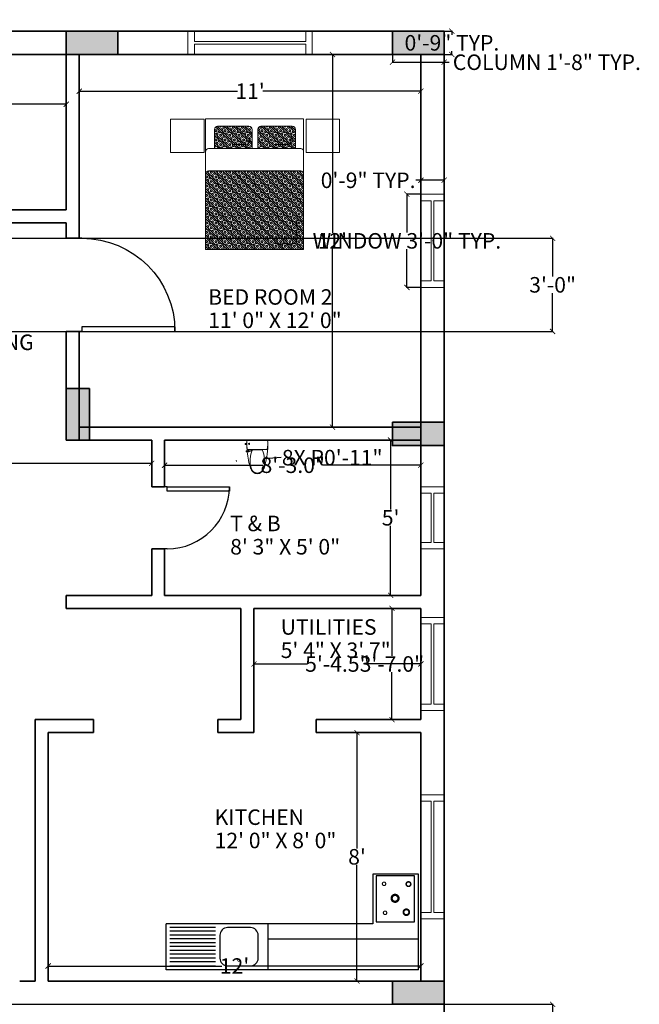
# Model space of a CAD drawing. Units: inches. Extents: x 560 to 1118, y 291 to 1226.
# Tile 4 of 4: x 878 to 1118, y 804 to 1184. Entities that reach past the tile are written whole.
import ezdxf

# ---------------------------------------------------------------- set-up
doc = ezdxf.new("R2010")
doc.units = ezdxf.units.IN
doc.header["$MEASUREMENT"] = 0
for name, color, linetype, lineweight in [('A-ANNO-DIMS', 2, 'Continuous', 13), ('A-AREA-IDEN', 7, 'Continuous', 18), ('A-COLS', 7, 'Continuous', 35), ('A-FLOR-FIXT', 9, 'Continuous', 18), ('DOORS', 4, 'Continuous', 25), ('FURNITURE', 8, 'Continuous', 18), ('WALL', 7, 'Continuous', 35), ('WINDOWS', 80, 'Continuous', 18)]:
    doc.layers.add(name, color=color, linetype=linetype, lineweight=lineweight)
doc.layers.add('DUVAR', color=7, linetype='Continuous')
doc.layers.add('TEFRIS', color=11, linetype='Continuous')
doc.styles.get("Standard").update_dxf_attribs({"font": 'arial.ttf'})
doc.dimstyles.get("Standard").update_dxf_attribs({"dimtxt": 6, "dimasz": 2, "dimexe": 0.18, "dimexo": 0.0625, "dimgap": 0.09, "dimtad": 0, "dimtih": 1, "dimtoh": 1, "dimdec": 1, "dimzin": 0, "dimdsep": 46, "dimlunit": 3, "dimtxsty": 'Standard', "dimblk": 'ARCHTICK', "dimcen": 0.09, "dimadec": 0, "dimazin": 0, "dimtfac": 1, "dimtdec": 1, "dimtofl": 0, "dimtmove": 0, "dimatfit": 3, "dimfxl": 1, "dimtolj": 1, "dimtzin": 0, "dimarcsym": 0})
pattern_1 = [(135, (-1377.70473, -125.71507), (-0.070710678, -0.070710678), []), (135, (-1377.68705, -125.69739), (-0.070710678, -0.070710678), []), (45, (-1377.70473, -125.71507), (-0.070710678, 0.070710678), [-0.025, 0.025]), (45, (-1377.72241, -125.69739), (-0.070710678, 0.070710678), [-0.025, 0.025]), (45, (-1377.74009, -125.67972), (-0.070710678, 0.070710678), [0.025, -0.025]), (45, (-1377.75776, -125.66204), (-0.070710678, 0.070710678), [0.025, -0.025]), (135, (-1377.66938, -125.67972), (-0.070710678, -0.070710678), [0.025, -0.025]), (135, (-1377.6517, -125.66204), (-0.070710678, -0.070710678), [0.025, -0.025])]

# ---------------------------------------------------------------- blocks, each defined once
blk = doc.blocks.new('*U3')
for p, q in [((0, 0), (0, -6)), ((36, 0), (36, -6))]:
    blk.add_line(p, q)
blk.add_lwpolyline([(0, 0), (0, 36), (1.75, 36), (1.75, 0)], close=True)
blk.add_arc((0, 0), 36, 0, 90)
blk = doc.blocks.new('*U4')
for p, q in [((0, 0), (0, -6)), ((24, 0), (24, -6))]:
    blk.add_line(p, q)
blk.add_lwpolyline([(0, 0), (0, 24), (1.75, 24), (1.75, 0)], close=True)
blk.add_arc((0, 0), 24, 0, 90)
blk = doc.blocks.new('_ArchTick')
at = {"color": 0, "linetype": 'ByBlock', "const_width": 0.15}
blk.add_lwpolyline([(-0.5, -0.5), (0.5, 0.5)], dxfattribs=at)
blk = doc.blocks.new('*D8')
at = {"layer": 'A-ANNO-DIMS', "color": 0, "lineweight": -2, "transparency": 16777216}
for p, q in [((761.18, 1149.36), (761.18, 1151.98)), ((761.18, 1151.8), (815.07, 1151.8)), ((896.18, 1151.8), (842.29, 1151.8)), ((896.18, 1149.36), (896.18, 1151.98))]:
    blk.add_line(p, q, dxfattribs=at)
at = {"layer": 'Defpoints', "color": 0, "transparency": 16777216}
for p in [(761.18, 1149.3), (896.18, 1151.8), (896.18, 1149.3)]:
    blk.add_point(p, dxfattribs=at)
at = {"layer": 'A-ANNO-DIMS', "color": 0, "lineweight": -2, "transparency": 16777216, "xscale": 2, "yscale": 2, "zscale": 2, "rotation": 180}
blk.add_blockref('_ArchTick', (761.18, 1151.8), dxfattribs=at)
at = {"layer": 'A-ANNO-DIMS', "color": 0, "lineweight": -2, "transparency": 16777216, "xscale": 2, "yscale": 2, "zscale": 2}
blk.add_blockref('_ArchTick', (896.18, 1151.8), dxfattribs=at)
at = {"layer": 'A-ANNO-DIMS', "color": 0, "transparency": 16777216, "insert": (828.68, 1151.8), "char_height": 6, "attachment_point": 5}
blk.add_mtext('\\A1;11\'-3.0"', dxfattribs=at)
blk = doc.blocks.new('*D10')
at = {"layer": 'A-ANNO-DIMS', "color": 0, "lineweight": -2, "transparency": 16777216}
for p, q in [((1001.94, 1171), (998.82, 1171)), ((999, 1171), (999, 1102.1)), ((999, 1027), (999, 1095.9)), ((1001.94, 1027), (998.82, 1027))]:
    blk.add_line(p, q, dxfattribs=at)
at = {"layer": 'Defpoints', "color": 0, "transparency": 16777216}
for p in [(1002, 1171), (999, 1027), (1002, 1027)]:
    blk.add_point(p, dxfattribs=at)
at = {"layer": 'A-ANNO-DIMS', "color": 0, "lineweight": -2, "transparency": 16777216, "xscale": 2, "yscale": 2, "zscale": 2}
for p, rotation in [((999, 1171), 90), ((999, 1027), 270)]:
    blk.add_blockref('_ArchTick', p, dxfattribs=dict(at, rotation=rotation))
at = {"layer": 'A-ANNO-DIMS', "color": 0, "transparency": 16777216, "insert": (999, 1099), "char_height": 6, "attachment_point": 5}
blk.add_mtext("\\A1;12'", dxfattribs=at)
blk = doc.blocks.new('*D11')
at = {"layer": 'A-ANNO-DIMS', "color": 0, "lineweight": -2, "transparency": 16777216}
for p, q in [((901.18, 1165.24), (901.18, 1156.62)), ((1033.18, 1165.24), (1033.18, 1156.62)), ((901.18, 1156.8), (962.28, 1156.8)), ((1033.18, 1156.8), (972.08, 1156.8))]:
    blk.add_line(p, q, dxfattribs=at)
at = {"layer": 'Defpoints', "color": 0, "transparency": 16777216}
for p in [(901.18, 1165.3), (1033.18, 1165.3), (1033.18, 1156.8)]:
    blk.add_point(p, dxfattribs=at)
at = {"layer": 'A-ANNO-DIMS', "color": 0, "lineweight": -2, "transparency": 16777216, "xscale": 2, "yscale": 2, "zscale": 2, "rotation": 180}
blk.add_blockref('_ArchTick', (901.18, 1156.8), dxfattribs=at)
at = {"layer": 'A-ANNO-DIMS', "color": 0, "lineweight": -2, "transparency": 16777216, "xscale": 2, "yscale": 2, "zscale": 2}
blk.add_blockref('_ArchTick', (1033.18, 1156.8), dxfattribs=at)
at = {"layer": 'A-ANNO-DIMS', "color": 0, "transparency": 16777216, "insert": (967.18, 1156.8), "char_height": 6, "attachment_point": 5}
blk.add_mtext("\\A1;11'", dxfattribs=at)
blk = doc.blocks.new('*D14')
at = {"layer": 'A-ANNO-DIMS', "color": 0, "lineweight": -2, "transparency": 16777216}
for p, q in [((934.18, 1011.86), (934.18, 1012.48)), ((934.18, 1012.3), (972.12, 1012.3)), ((1033.18, 1012.3), (995.24, 1012.3)), ((1033.18, 1011.86), (1033.18, 1012.48))]:
    blk.add_line(p, q, dxfattribs=at)
at = {"layer": 'Defpoints', "color": 0, "transparency": 16777216}
for p in [(934.18, 1012.3), (934.18, 1011.8), (1033.18, 1011.8)]:
    blk.add_point(p, dxfattribs=at)
at = {"layer": 'A-ANNO-DIMS', "color": 0, "lineweight": -2, "transparency": 16777216, "xscale": 2, "yscale": 2, "zscale": 2, "rotation": 180}
blk.add_blockref('_ArchTick', (934.18, 1012.3), dxfattribs=at)
at = {"layer": 'A-ANNO-DIMS', "color": 0, "lineweight": -2, "transparency": 16777216, "xscale": 2, "yscale": 2, "zscale": 2}
blk.add_blockref('_ArchTick', (1033.18, 1012.3), dxfattribs=at)
at = {"layer": 'A-ANNO-DIMS', "color": 0, "transparency": 16777216, "insert": (983.68, 1012.3), "char_height": 6, "attachment_point": 5}
blk.add_mtext('\\A1;8\'-3.0"', dxfattribs=at)
blk = doc.blocks.new('*D15')
at = {"layer": 'A-ANNO-DIMS', "color": 0, "lineweight": -2, "transparency": 16777216}
for p, q in [((1018.56, 1022), (1021.68, 1022)), ((1021.5, 1022), (1021.5, 995.14)), ((1021.5, 962), (1021.5, 988.86)), ((1018.56, 962), (1021.68, 962))]:
    blk.add_line(p, q, dxfattribs=at)
at = {"layer": 'Defpoints', "color": 0, "transparency": 16777216}
for p in [(1018.5, 1022), (1018.5, 962), (1021.5, 962)]:
    blk.add_point(p, dxfattribs=at)
at = {"layer": 'A-ANNO-DIMS', "color": 0, "lineweight": -2, "transparency": 16777216, "xscale": 2, "yscale": 2, "zscale": 2}
for p, rotation in [((1021.5, 1022), 90), ((1021.5, 962), 270)]:
    blk.add_blockref('_ArchTick', p, dxfattribs=dict(at, rotation=rotation))
at = {"layer": 'A-ANNO-DIMS', "color": 0, "transparency": 16777216, "insert": (1021.5, 992), "char_height": 6, "attachment_point": 5}
blk.add_mtext("\\A1;5'", dxfattribs=at)
blk = doc.blocks.new('*D34')
at = {"layer": 'A-ANNO-DIMS', "color": 0, "lineweight": -2, "transparency": 16777216}
for p, q in [((889.18, 818.86), (889.18, 818.98)), ((889.18, 818.8), (956.28, 818.8)), ((1033.18, 818.8), (966.08, 818.8)), ((1033.18, 818.86), (1033.18, 818.98))]:
    blk.add_line(p, q, dxfattribs=at)
at = {"layer": 'Defpoints', "color": 0, "transparency": 16777216}
for p in [(889.18, 818.8), (1033.18, 818.8), (1033.18, 818.8)]:
    blk.add_point(p, dxfattribs=at)
at = {"layer": 'A-ANNO-DIMS', "color": 0, "lineweight": -2, "transparency": 16777216, "xscale": 2, "yscale": 2, "zscale": 2, "rotation": 180}
blk.add_blockref('_ArchTick', (889.18, 818.8), dxfattribs=at)
at = {"layer": 'A-ANNO-DIMS', "color": 0, "lineweight": -2, "transparency": 16777216, "xscale": 2, "yscale": 2, "zscale": 2}
blk.add_blockref('_ArchTick', (1033.18, 818.8), dxfattribs=at)
at = {"layer": 'A-ANNO-DIMS', "color": 0, "transparency": 16777216, "insert": (961.18, 818.8), "char_height": 6, "attachment_point": 5}
blk.add_mtext("\\A1;12'", dxfattribs=at)
blk = doc.blocks.new('*D35')
at = {"layer": 'A-ANNO-DIMS', "color": 0, "lineweight": -2, "transparency": 16777216}
for p, q in [((1008.5, 909), (1008.5, 864.15)), ((1008.56, 909), (1008.68, 909)), ((1008.5, 813), (1008.5, 857.85)), ((1008.56, 813), (1008.68, 813))]:
    blk.add_line(p, q, dxfattribs=at)
at = {"layer": 'Defpoints', "color": 0, "transparency": 16777216}
for p in [(1008.5, 909), (1008.5, 813), (1008.5, 813)]:
    blk.add_point(p, dxfattribs=at)
at = {"layer": 'A-ANNO-DIMS', "color": 0, "lineweight": -2, "transparency": 16777216, "xscale": 2, "yscale": 2, "zscale": 2}
for p, rotation in [((1008.5, 909), 90), ((1008.5, 813), 270)]:
    blk.add_blockref('_ArchTick', p, dxfattribs=dict(at, rotation=rotation))
at = {"layer": 'A-ANNO-DIMS', "color": 0, "transparency": 16777216, "insert": (1008.5, 861), "char_height": 6, "attachment_point": 5}
blk.add_mtext("\\A1;8'", dxfattribs=at)
blk = doc.blocks.new('*D36')
at = {"layer": 'A-ANNO-DIMS', "color": 0, "lineweight": -2, "transparency": 16777216}
for p, q in [((968.68, 935.56), (968.68, 935.68)), ((968.68, 935.5), (989.37, 935.5)), ((1033.18, 935.5), (1012.49, 935.5)), ((1033.18, 935.56), (1033.18, 935.68))]:
    blk.add_line(p, q, dxfattribs=at)
at = {"layer": 'Defpoints', "color": 0, "transparency": 16777216}
for p in [(968.68, 935.5), (1033.18, 935.5), (1033.18, 935.5)]:
    blk.add_point(p, dxfattribs=at)
at = {"layer": 'A-ANNO-DIMS', "color": 0, "lineweight": -2, "transparency": 16777216, "xscale": 2, "yscale": 2, "zscale": 2, "rotation": 180}
blk.add_blockref('_ArchTick', (968.68, 935.5), dxfattribs=at)
at = {"layer": 'A-ANNO-DIMS', "color": 0, "lineweight": -2, "transparency": 16777216, "xscale": 2, "yscale": 2, "zscale": 2}
blk.add_blockref('_ArchTick', (1033.18, 935.5), dxfattribs=at)
at = {"layer": 'A-ANNO-DIMS', "color": 0, "transparency": 16777216, "insert": (1000.93, 935.5), "char_height": 6, "attachment_point": 5}
blk.add_mtext('\\A1;5\'-4.5"', dxfattribs=at)
blk = doc.blocks.new('*D37')
at = {"layer": 'A-ANNO-DIMS', "color": 0, "lineweight": -2, "transparency": 16777216}
for p, q in [((1020.06, 957), (1022.18, 957)), ((1022, 957), (1022, 938.66)), ((1022, 914), (1022, 932.34)), ((1020.06, 914), (1022.18, 914))]:
    blk.add_line(p, q, dxfattribs=at)
at = {"layer": 'Defpoints', "color": 0, "transparency": 16777216}
for p in [(1020, 957), (1020, 914), (1022, 914)]:
    blk.add_point(p, dxfattribs=at)
at = {"layer": 'A-ANNO-DIMS', "color": 0, "lineweight": -2, "transparency": 16777216, "xscale": 2, "yscale": 2, "zscale": 2}
for p, rotation in [((1022, 957), 90), ((1022, 914), 270)]:
    blk.add_blockref('_ArchTick', p, dxfattribs=dict(at, rotation=rotation))
at = {"layer": 'A-ANNO-DIMS', "color": 0, "transparency": 16777216, "insert": (1022, 935.5), "char_height": 6, "attachment_point": 5}
blk.add_mtext('\\A1;3\'-7.0"', dxfattribs=at)
blk = doc.blocks.new('*D39')
at = {"layer": 'A-ANNO-DIMS', "color": 0, "lineweight": -2, "transparency": 16777216}
for p, q in [((728.18, 1015.74), (728.18, 1012.82)), ((728.18, 1013), (815.07, 1013)), ((929.18, 1013), (842.29, 1013)), ((929.18, 1015.74), (929.18, 1012.82))]:
    blk.add_line(p, q, dxfattribs=at)
at = {"layer": 'Defpoints', "color": 0, "transparency": 16777216}
for p in [(728.18, 1015.8), (929.18, 1015.8), (929.18, 1013)]:
    blk.add_point(p, dxfattribs=at)
at = {"layer": 'A-ANNO-DIMS', "color": 0, "lineweight": -2, "transparency": 16777216, "xscale": 2, "yscale": 2, "zscale": 2, "rotation": 180}
blk.add_blockref('_ArchTick', (728.18, 1013), dxfattribs=at)
at = {"layer": 'A-ANNO-DIMS', "color": 0, "lineweight": -2, "transparency": 16777216, "xscale": 2, "yscale": 2, "zscale": 2}
blk.add_blockref('_ArchTick', (929.18, 1013), dxfattribs=at)
at = {"layer": 'A-ANNO-DIMS', "color": 0, "transparency": 16777216, "insert": (828.68, 1013), "char_height": 6, "attachment_point": 5}
blk.add_mtext('\\A1;16\'-9.0"', dxfattribs=at)
blk = doc.blocks.new('MAT-P10')
h = blk.add_hatch()
h.set_pattern_fill('BOX', color=256, scale=0.1, angle=45, style=0)
h.set_pattern_definition(pattern_1)
h.paths.add_polyline_path([(-0.157, 1.46), (0.417, 1.46), (0.417, 1.751, 0.414214), (0.367, 1.801), (-0.107, 1.801, 0.414214), (-0.157, 1.751)])
h.paths.add_polyline_path([(0.505, 1.46), (1.079, 1.46), (1.079, 1.751, 0.414214), (1.029, 1.801), (0.555, 1.801, 0.414214), (0.505, 1.751)])
h = blk.add_hatch()
h.set_pattern_fill('BOX', color=256, scale=0.1, angle=45, style=0)
h.set_pattern_definition(pattern_1)
edge = h.paths.add_edge_path()
edge.add_line((1.205, -0.085), (1.205, 1.062))
edge.add_ellipse((1.161, 1.063), major_axis=(0, 0.0568), ratio=0.776379, start_angle=270, end_angle=360)
edge.add_line((1.161, 1.119), (-0.251, 1.12))
edge.add_ellipse((-0.251, 1.063), major_axis=(0, 0.0568), ratio=0.776379, start_angle=0, end_angle=88.1396)
edge.add_line((-0.295, 1.064), (-0.295, -0.085))
edge.add_line((-0.295, -0.085), (1.205, -0.085))
for p, q in [((-0.251, 1.46), (1.161, 1.46)), ((-0.251, 1.12), (1.161, 1.119)), ((1.102, 0.406), (1.102, 0.057)), ((1.058, 0), (0.775, 0))]:
    blk.add_line(p, q)
for points in [[(-0.83, 1.909), (-0.319, 1.909), (-0.319, 1.398), (-0.83, 1.398)], [(1.205, -0.085), (-0.295, -0.085), (-0.295, 1.915), (1.205, 1.915)], [(1.244, 1.909), (1.755, 1.909), (1.755, 1.398), (1.244, 1.398)]]:
    blk.add_lwpolyline(points, close=True)
for points in [[(0.417, 1.46), (0.417, 1.751, 0.414214), (0.367, 1.801), (-0.107, 1.801, 0.414214), (-0.157, 1.751), (-0.157, 1.46)], [(1.079, 1.46), (1.079, 1.751, 0.414214), (1.029, 1.801), (0.555, 1.801, 0.414214), (0.505, 1.751), (0.505, 1.46)], [(0.37, 1.624), (0.37, 1.571, -0.414214), (0.32, 1.521), (0.111, 1.521)], [(1.012, 1.644), (1.012, 1.571, -0.414214), (0.962, 1.521), (0.753, 1.521)]]:
    blk.add_lwpolyline(points, format="xyb")
at = {"extrusion": (0, 0, -1)}
for centre, start_param, end_param in [((-0.251, 1.404), 4.712389, 6.283185), ((1.161, 1.404), 0, 1.570796), ((-0.251, 1.063), 4.712389, 6.283185), ((1.161, 1.063), 0, 1.570796), ((1.058, 0.057), 1.570796, 3.141593), ((1.058, 0.057), 1.570796, 3.141593)]:
    blk.add_ellipse(centre, major_axis=(0, 0.0568), ratio=0.776379, start_param=start_param, end_param=end_param, dxfattribs=at)
blk = doc.blocks.new('A$C3F871443')
at = {"layer": 'DUVAR'}
blk.add_line((3, 0), (3.3, 0), dxfattribs=at)
at = {"layer": 'TEFRIS'}
for p, q in [((0, 0), (0, -1.25)), ((0, 0), (3.3, 0)), ((1.97, -0.6), (1.97, 0)), ((3.3, 0), (3.3, -0.6)), ((3.253, -0.055), (2.653, -0.055)), ((2.653, -0.105), (3.253, -0.105)), ((2.653, -0.155), (3.253, -0.155)), ((2.653, -0.205), (3.253, -0.205)), ((2.653, -0.255), (3.253, -0.255)), ((2.653, -0.305), (3.253, -0.305)), ((2.653, -0.355), (3.253, -0.355)), ((0, -0.4), (1.97, -0.4)), ((2.653, -0.405), (3.253, -0.405)), ((2.653, -0.455), (3.253, -0.455)), ((2.653, -0.505), (3.253, -0.505)), ((0.6, -0.6), (3.3, -0.6)), ((0.6, -1.25), (0.6, -0.6)), ((2.653, -0.555), (3.253, -0.555)), ((0, -1.25), (0.6, -1.25))]:
    blk.add_line(p, q, dxfattribs=at)
blk.add_lwpolyline([(2.597, -0.452), (2.597, -0.152, 0.414214), (2.497, -0.052), (2.197, -0.052, 0.414214), (2.097, -0.152), (2.097, -0.452, 0.414214), (2.197, -0.552), (2.497, -0.552, 0.414214)], format="xyb", close=True, dxfattribs=at)
for points, const_width in [([(2.349, -0.141, 1), (2.349, -0.111, 1)], 0.01), ([(0.161, -0.791, 1), (0.161, -0.716, 1)], 0.025), ([(0.439, -0.768, 1), (0.439, -0.723, 1)], 0.015), ([(0.308, -0.98, 1), (0.308, -0.89, 1)], 0.03), ([(0.133, -1.151, 1), (0.133, -1.091, 1)], 0.02), ([(0.452, -1.147, 1), (0.452, -1.102, 1)], 0.015)]:
    blk.add_lwpolyline(points, format="xyb", close=True, dxfattribs=dict(at, const_width=const_width))
blk.add_lwpolyline([(0.556, -1.228), (0.556, -0.628), (0.056, -0.628), (0.056, -1.228)], close=True, dxfattribs=at)
blk = doc.blocks.new('toilet-7')
at = {"color": 0, "linetype": 'ByBlock'}
for p, q in [((-0.246, -0.087), (-0.246, -0.107)), ((-0.246, -0.087), (-0.226, -0.087)), ((-0.246, -0.107), (-0.226, -0.107)), ((-0.226, -0.085), (-0.226, -0.11)), ((-0.226, -0.085), (-0.216, -0.085)), ((-0.226, -0.11), (-0.215, -0.11)), ((0.21, -0.02), (-0.21, -0.02)), ((0.199, -0.212), (0.21, -0.164)), ((0.215, -0.068), (0.21, -0.02)), ((0.21, -0.164), (0.215, -0.117)), ((0.215, -0.117), (0.215, -0.068)), ((-0.121, -0.237), (-0.228, -0.237)), ((-0.228, -0.237), (-0.228, -0.26)), ((-0.176, -0.26), (-0.228, -0.26)), ((0.199, -0.212), (-0.199, -0.212)), ((-0.18, -0.237), (-0.18, -0.212)), ((-0.176, -0.26), (-0.138, -0.245)), ((-0.138, -0.245), (-0.138, -0.237)), ((-0.121, -0.237), (-0.121, -0.212)), ((-0.102, -0.221), (0.102, -0.221))]:
    blk.add_line(p, q, dxfattribs=at)
blk.add_circle((-0.17, -0.097), 0.0125, dxfattribs=at)
for centre, radius, start, end in [((0.224, -0.092), 0.44, 170.5377, 187.7399), ((1.517, -0.087), 1.732, 181.2224, 184.9822), ((0.224, -0.092), 0.44, 187.7399, 195.822), ((-1.517, -0.087), 1.732, 342.7523, 358.7776), ((1.517, -0.087), 1.732, 185.7323, 197.2477), ((0.426, -0.441), 0.572, 157.3737, 194.7786), ((-0.426, -0.441), 0.572, 345.2214, 22.6263), ((0.012, -0.554), 0.155, 197.2477, 249.5476), ((0.022, -0.548), 0.155, 194.7786, 226.8543), ((-0.012, -0.554), 0.155, 290.4524, 342.7523), ((-0.022, -0.548), 0.155, 313.1457, 345.2214), ((0, -0.571), 0.122, 226.8543, 313.1457), ((0, -0.585), 0.122, 249.5476, 290.4524)]:
    blk.add_arc(centre, radius, start, end, dxfattribs=at)
blk = doc.blocks.new('WIN-48IN')
for p, q in [((0, 9), (48, 9)), ((0, 0), (0, 9)), ((2.5, 5), (2.5, 9)), ((45.5, 9), (45.5, 5)), ((48, 9), (48, 0)), ((2.5, 5), (45.5, 5)), ((2.5, 0), (2.5, 4)), ((2.5, 4), (45.5, 4)), ((45.5, 4), (45.5, 0)), ((48, 0), (0, 0))]:
    blk.add_line(p, q)
blk = doc.blocks.new('WIN-36IN')
for p, q in [((0, 0), (0, 36)), ((0, 36), (9, 36)), ((9, 36), (9, 0)), ((0, 33.5), (4, 33.5)), ((4, 33.5), (4, 2.5)), ((5, 33.5), (9, 33.5)), ((5, 33.5), (5, 2.5)), ((4, 2.5), (0, 2.5)), ((9, 0), (0, 0)), ((9, 2.5), (5, 2.5))]:
    blk.add_line(p, q)
blk = doc.blocks.new('WIN-24IN')
for p, q in [((0, 0), (0, 24)), ((0, 24), (9, 24)), ((9, 24), (9, 0)), ((0, 21.5), (4, 21.5)), ((4, 21.5), (4, 2.5)), ((5, 21.5), (9, 21.5)), ((5, 21.5), (5, 2.5)), ((4, 2.5), (0, 2.5)), ((9, 0), (0, 0)), ((9, 2.5), (5, 2.5))]:
    blk.add_line(p, q)
blk = doc.blocks.new('COL-RECT-9X20-NOM')
h = blk.add_hatch(color=256)
h.dxf.hatch_style = 1
h.paths.add_polyline_path([(19.98, 0), (19.98, 9), (0, 9), (0, 0)])
blk.add_lwpolyline([(0, 9), (0, 0), (19.98, 0), (19.98, 9)], close=True)
blk = doc.blocks.new('*D57')
at = {"layer": 'A-ANNO-DIMS', "color": 0, "lineweight": -2, "transparency": 16777216}
for p, q in [((1022.2, 1170.94), (1022.2, 1167.82)), ((1022.2, 1168), (1042.18, 1168)), ((1042.18, 1170.94), (1042.18, 1167.82)), ((1042.18, 1168), (1044.18, 1168))]:
    blk.add_line(p, q, dxfattribs=at)
at = {"layer": 'Defpoints', "color": 0, "transparency": 16777216}
for p in [(1022.2, 1171), (1042.18, 1171), (1042.18, 1168)]:
    blk.add_point(p, dxfattribs=at)
at = {"layer": 'A-ANNO-DIMS', "color": 0, "lineweight": -2, "transparency": 16777216, "xscale": 2, "yscale": 2, "zscale": 2, "rotation": 180}
blk.add_blockref('_ArchTick', (1022.2, 1168), dxfattribs=at)
at = {"layer": 'A-ANNO-DIMS', "color": 0, "lineweight": -2, "transparency": 16777216, "xscale": 2, "yscale": 2, "zscale": 2}
blk.add_blockref('_ArchTick', (1042.18, 1168), dxfattribs=at)
at = {"layer": 'A-ANNO-DIMS', "color": 0, "transparency": 16777216, "insert": (1081.85, 1168), "char_height": 6, "attachment_point": 5}
blk.add_mtext('\\A1;COLUMN 1\'-8" TYP.', dxfattribs=at)
blk = doc.blocks.new('*D58')
at = {"layer": 'A-ANNO-DIMS', "color": 0, "lineweight": -2, "transparency": 16777216}
for p, q in [((1042.24, 1180), (1045.36, 1180)), ((1045.18, 1180), (1045.18, 1178.65)), ((1045.18, 1171), (1045.18, 1172.35)), ((1042.24, 1171), (1045.36, 1171))]:
    blk.add_line(p, q, dxfattribs=at)
at = {"layer": 'Defpoints', "color": 0, "transparency": 16777216}
for p in [(1042.18, 1180), (1045.18, 1180), (1042.18, 1171)]:
    blk.add_point(p, dxfattribs=at)
at = {"layer": 'A-ANNO-DIMS', "color": 0, "lineweight": -2, "transparency": 16777216, "xscale": 2, "yscale": 2, "zscale": 2}
for p, rotation in [((1045.18, 1180), 90), ((1045.18, 1171), 270)]:
    blk.add_blockref('_ArchTick', p, dxfattribs=dict(at, rotation=rotation))
at = {"layer": 'A-ANNO-DIMS', "color": 0, "transparency": 16777216, "insert": (1045.18, 1175.5), "char_height": 6, "attachment_point": 5}
blk.add_mtext('\\A1;0\'-9" TYP.', dxfattribs=at)
blk = doc.blocks.new('*D63')
at = {"layer": 'A-ANNO-DIMS', "color": 0, "lineweight": -2, "transparency": 16777216}
for p, q in [((1033.12, 1117), (1027.6, 1117)), ((1027.78, 1117), (1027.78, 1102.2)), ((1027.78, 1081), (1027.78, 1095.8)), ((1033.12, 1081), (1027.6, 1081))]:
    blk.add_line(p, q, dxfattribs=at)
at = {"layer": 'Defpoints', "color": 0, "transparency": 16777216}
for p in [(1033.18, 1117), (1027.78, 1081), (1033.18, 1081)]:
    blk.add_point(p, dxfattribs=at)
at = {"layer": 'A-ANNO-DIMS', "color": 0, "lineweight": -2, "transparency": 16777216, "xscale": 2, "yscale": 2, "zscale": 2}
for p, rotation in [((1027.78, 1117), 90), ((1027.78, 1081), 270)]:
    blk.add_blockref('_ArchTick', p, dxfattribs=dict(at, rotation=rotation))
at = {"layer": 'A-ANNO-DIMS', "color": 0, "transparency": 16777216, "insert": (1027.78, 1099), "char_height": 6, "attachment_point": 5}
blk.add_mtext('\\A1;WINDOW 3\'-0" TYP.', dxfattribs=at)
blk = doc.blocks.new('*D64')
at = {"layer": 'A-ANNO-DIMS', "color": 0, "lineweight": -2, "transparency": 16777216}
for p, q in [((1033.18, 1122.4), (1031.18, 1122.4)), ((1033.18, 1117.06), (1033.18, 1122.58)), ((1042.18, 1122.4), (1033.18, 1122.4)), ((1042.18, 1117.06), (1042.18, 1122.58))]:
    blk.add_line(p, q, dxfattribs=at)
at = {"layer": 'Defpoints', "color": 0, "transparency": 16777216}
for p in [(1033.18, 1122.4), (1033.18, 1117), (1042.18, 1117)]:
    blk.add_point(p, dxfattribs=at)
at = {"layer": 'A-ANNO-DIMS', "color": 0, "lineweight": -2, "transparency": 16777216, "xscale": 2, "yscale": 2, "zscale": 2, "rotation": 180}
blk.add_blockref('_ArchTick', (1033.18, 1122.4), dxfattribs=at)
at = {"layer": 'A-ANNO-DIMS', "color": 0, "lineweight": -2, "transparency": 16777216, "xscale": 2, "yscale": 2, "zscale": 2}
blk.add_blockref('_ArchTick', (1042.18, 1122.4), dxfattribs=at)
at = {"layer": 'A-ANNO-DIMS', "color": 0, "transparency": 16777216, "insert": (1012.8, 1122.4), "char_height": 6, "attachment_point": 5}
blk.add_mtext('\\A1;0\'-9" TYP.', dxfattribs=at)
blk = doc.blocks.new('*D73')
at = {"layer": 'A-ANNO-DIMS', "color": 0, "lineweight": -2, "transparency": 16777216}
for p, q in [((756.24, 1100), (1084.26, 1100)), ((1084.08, 1100), (1084.08, 1085.16)), ((1084.08, 1064), (1084.08, 1078.84)), ((756.24, 1064), (1084.26, 1064))]:
    blk.add_line(p, q, dxfattribs=at)
at = {"layer": 'Defpoints', "color": 0, "transparency": 16777216}
for p in [(756.18, 1100), (1084.08, 1100), (756.18, 1064)]:
    blk.add_point(p, dxfattribs=at)
at = {"layer": 'A-ANNO-DIMS', "color": 0, "lineweight": -2, "transparency": 16777216, "xscale": 2, "yscale": 2, "zscale": 2}
for p, rotation in [((1084.08, 1100), 90), ((1084.08, 1064), 270)]:
    blk.add_blockref('_ArchTick', p, dxfattribs=dict(at, rotation=rotation))
at = {"layer": 'A-ANNO-DIMS', "color": 0, "transparency": 16777216, "insert": (1084.08, 1082), "char_height": 6, "attachment_point": 5}
blk.add_mtext('\\A1;3\'-0"', dxfattribs=at)
blk = doc.blocks.new('*D78')
at = {"layer": 'A-ANNO-DIMS', "color": 0, "lineweight": -2, "transparency": 16777216}
for p, q in [((794.7, 804), (1084.26, 804)), ((1084.08, 804), (1084.08, 789.16)), ((1084.08, 768), (1084.08, 782.84)), ((794.7, 768), (1084.26, 768))]:
    blk.add_line(p, q, dxfattribs=at)
at = {"layer": 'Defpoints', "color": 0, "transparency": 16777216}
for p in [(794.64, 804), (1084.08, 804), (794.64, 768)]:
    blk.add_point(p, dxfattribs=at)
at = {"layer": 'A-ANNO-DIMS', "color": 0, "lineweight": -2, "transparency": 16777216, "xscale": 2, "yscale": 2, "zscale": 2}
for p, rotation in [((1084.08, 804), 90), ((1084.08, 768), 270)]:
    blk.add_blockref('_ArchTick', p, dxfattribs=dict(at, rotation=rotation))
at = {"layer": 'A-ANNO-DIMS', "color": 0, "transparency": 16777216, "insert": (1084.08, 786), "char_height": 6, "attachment_point": 5}
blk.add_mtext('\\A1;3\'-0"', dxfattribs=at)
blk = doc.blocks.new('*D81')
at = {"layer": 'A-ANNO-DIMS', "color": 0, "lineweight": -2, "transparency": 16777216}
for p, q in [((961.86, 1014.04), (962.04, 1014.04)), ((961.95, 1013.95), (961.95, 1014.13)), ((979.21, 1015.22), (972.74, 1014.78))]:
    blk.add_line(p, q, dxfattribs=at)
at = {"layer": 'Defpoints', "color": 0, "transparency": 16777216}
for p in [(961.95, 1014.04), (972.74, 1014.78)]:
    blk.add_point(p, dxfattribs=at)
at = {"layer": 'A-ANNO-DIMS', "color": 0, "lineweight": -2, "transparency": 16777216, "xscale": 2, "yscale": 2, "zscale": 2, "rotation": 183.9218187656538}
blk.add_blockref('_ArchTick', (972.74, 1014.78), dxfattribs=at)
at = {"layer": 'A-ANNO-DIMS', "color": 0, "transparency": 16777216, "insert": (998.93, 1015.22), "char_height": 6, "attachment_point": 5}
blk.add_mtext('\\A1;8X R0\'-11"', dxfattribs=at)

msp = doc.modelspace()

# ---------------------------------------------------------------- linework, layer by layer
at = {"layer": 'WALL'}
for p, q in [((761.18, 1180), (896.18, 1180)), ((1042.18, 1180), (896.18, 1180)), ((896.18, 1180), (896.18, 1111)), ((1042.18, 1180), (1042.18, 342)), ((761.18, 1171), (896.18, 1171)), ((1033.18, 1171), (901.18, 1171)), ((901.18, 1171), (901.18, 1100)), ((1033.18, 1171), (1033.18, 1027)), ((1033.18, 1171), (1033.18, 1027)), ((896.18, 1111), (761.18, 1111)), ((896.18, 1106), (761.18, 1106)), ((896.18, 1106), (896.18, 1100)), ((896.18, 1100), (901.18, 1100)), ((896.18, 1064), (901.18, 1064)), ((896.18, 1064), (896.18, 1022)), ((901.18, 1064), (901.18, 1022)), ((1033.18, 1027), (901.18, 1027)), ((1033.18, 1027), (1033.18, 1022)), ((929.18, 1022), (896.18, 1022)), ((929.18, 1022), (929.18, 1004)), ((1033.18, 1022), (934.18, 1022)), ((934.18, 1022), (934.18, 1004)), ((1033.18, 1022), (1033.18, 962)), ((934.18, 1004), (929.18, 1004)), ((934.18, 980), (929.18, 980)), ((929.18, 980), (929.18, 962)), ((934.18, 980), (934.18, 962)), ((896.18, 962), (896.18, 957)), ((929.18, 962), (896.18, 962)), ((1033.18, 962), (934.18, 962)), ((963.68, 957), (896.18, 957)), ((963.68, 957), (963.68, 914)), ((1033.18, 957), (968.68, 957)), ((968.68, 957), (968.68, 914)), ((1033.18, 957), (1033.18, 914)), ((884.18, 909), (884.18, 914)), ((906.68, 914), (884.18, 914)), ((906.68, 914), (906.68, 909)), ((963.68, 914), (954.68, 914)), ((954.68, 914), (954.68, 909)), ((968.68, 914), (968.68, 909)), ((1033.18, 914), (992.68, 914)), ((992.68, 914), (992.68, 909)), ((884.18, 909), (884.18, 813)), ((889.18, 909), (889.18, 813)), ((906.68, 909), (889.18, 909)), ((968.68, 909), (954.68, 909)), ((1033.18, 909), (992.68, 909)), ((1033.18, 909), (1033.18, 813)), ((884.18, 813), (878.18, 813)), ((884.18, 813), (878.18, 813)), ((896.18, 813), (889.18, 813)), ((1033.18, 813), (896.18, 813))]:
    msp.add_line(p, q, dxfattribs=at)

# ---------------------------------------------------------------- block references
at = {"layer": 'A-COLS'}
for p in [(896.18, 1171), (1022.2, 1171), (1022.2, 1019.9), (1022.2, 804)]:
    msp.add_blockref('COL-RECT-9X20-NOM', p, dxfattribs=at)
at = {"layer": 'A-COLS', "rotation": 270.0000000000001}
msp.add_blockref('COL-RECT-9X20-NOM', (896.18, 1041.98), dxfattribs=at)
at = {"layer": 'A-FLOR-FIXT', "xscale": 18.9039470471375, "yscale": 18.9039470471375, "zscale": 18.9039470471375}
msp.add_blockref('toilet-7', (970, 1022.38), dxfattribs=at)
at = {"layer": 'A-FLOR-FIXT', "xscale": 29.57142857142857, "yscale": 29.57142857142857, "zscale": 29.57142857142857, "rotation": 180}
msp.add_blockref('A$C3F871443', (1032.33, 817.3), dxfattribs=at)
at = {"layer": 'DOORS', "xscale": -1, "rotation": 269.9999999999994}
msp.add_blockref('*U3', (902.18, 1064), dxfattribs=at)
at = {"layer": 'DOORS', "rotation": 270}
msp.add_blockref('*U4', (935.18, 1004), dxfattribs=at)
at = {"layer": 'FURNITURE', "xscale": 25.25, "yscale": 25.25, "zscale": 25.25}
msp.add_blockref('MAT-P10', (957.46, 1097.82), dxfattribs=at)
at = {"layer": 'WINDOWS'}
msp.add_blockref('WIN-48IN', (943.18, 1171), dxfattribs=at)
for name, p, rotation in [('WIN-36IN', (1042.18, 1117), 180), ('WIN-24IN', (1042.18, 1004), 180), ('WIN-36IN', (1042.18, 953.5), 180), ('WIN-48IN', (1033.18, 885), 270)]:
    msp.add_blockref(name, p, dxfattribs=dict(at, rotation=rotation))

# ---------------------------------------------------------------- texts
at = {"layer": 'A-AREA-IDEN'}
for s, p in [('BED ROOM 2', (951, 1074.3)), ('11\' 0" X 12\' 0"', (951, 1065.3)), ('LIVING AND DINING', (810, 1056.8)), ('T & B', (959.5, 986.8)), ('8\' 3" X 5\' 0"', (959.5, 977.8)), ('UTILITIES', (979.02, 946.8)), ('5\' 4" X 3\' 7"', (979.02, 937.8)), ('KITCHEN', (953.5, 873.3)), ('12\' 0" X 8\' 0"', (953.5, 864.3))]:
    msp.add_text(s, height=6, dxfattribs=at).set_placement(p)

# ---------------------------------------------------------------- dimensions: what is measured, and where the dimension line sits
at = {"layer": 'A-ANNO-DIMS'}
for base, p1, p2, angle, text, picture, middle in [((1045.18, 1180), (1042.18, 1171), (1042.18, 1180), 90, '<> TYP.', '*D58', (1045.18, 1175.5)), ((1033.18, 1122.4), (1042.18, 1117), (1033.18, 1117), 180, '<> TYP.', '*D64', (1012.8, 1122.4)), ((1027.78, 1081), (1033.18, 1117), (1033.18, 1081), 270, 'WINDOW <> TYP.', '*D63', (1027.78, 1099))]:
    dim = msp.add_linear_dim(base=base, p1=p1, p2=p2, angle=angle, text=text, dimstyle='Standard', override={"dimdec": 1, "dimlfac": 1, "dimrnd": 0, "dimzin": 1, "dimdsep": 46, "dimlunit": 4, "dimfrac": 2}, dxfattribs=at)
    dim.commit()
    dim.dimension.update_dxf_attribs({"geometry": picture, "text_midpoint": middle})
dim = msp.add_linear_dim(base=(1042.18, 1168), p1=(1022.2, 1171), p2=(1042.18, 1171), text='COLUMN <> TYP.', dimstyle='Standard', override={"dimdec": 1, "dimlfac": 1, "dimrnd": 0, "dimzin": 1, "dimdsep": 46, "dimlunit": 4, "dimfrac": 2}, dxfattribs=at)
dim.commit()
dim.dimension.update_dxf_attribs({"geometry": '*D57', "text_midpoint": (1081.85, 1168)})
for base, p1, p2, override, picture, middle in [((999, 1027), (1002, 1171), (1002, 1027), {"dimclrd": 0, "dimclre": 0, "dimclrt": 0}, '*D10', (999, 1099)), ((1084.08, 1100), (756.18, 1064), (756.18, 1100), {"dimdec": 1, "dimlfac": 1, "dimrnd": 0, "dimzin": 1, "dimdsep": 46, "dimlunit": 4, "dimfrac": 2}, '*D73', (1084.08, 1082)), ((1021.5, 962), (1018.5, 1022), (1018.5, 962), {"dimclrd": 0, "dimclre": 0, "dimclrt": 0}, '*D15', (1021.5, 992)), ((1022, 914), (1020, 957), (1020, 914), {"dimclrd": 0, "dimclre": 0, "dimclrt": 0}, '*D37', (1022, 935.5)), ((1008.5, 813), (1008.5, 909), (1008.5, 813), {"dimclrd": 0, "dimclre": 0, "dimclrt": 0}, '*D35', (1008.5, 861)), ((1084.08, 804), (794.64, 768), (794.64, 804), {"dimdec": 1, "dimlfac": 1, "dimrnd": 0, "dimzin": 1, "dimdsep": 46, "dimlunit": 4, "dimfrac": 2}, '*D78', (1084.08, 786))]:
    dim = msp.add_linear_dim(base=base, p1=p1, p2=p2, angle=90, dimstyle='Standard', override=override, dxfattribs=at)
    dim.commit()
    dim.dimension.update_dxf_attribs({"geometry": picture, "text_midpoint": middle})
for base, p1, p2, picture, middle in [((1033.18, 1156.8), (901.18, 1165.3), (1033.18, 1165.3), '*D11', (967.18, 1156.8)), ((896.18, 1151.8), (761.18, 1149.3), (896.18, 1149.3), '*D8', (828.68, 1151.8)), ((929.18, 1013), (728.18, 1015.8), (929.18, 1015.8), '*D39', (828.68, 1013)), ((934.18, 1012.3), (1033.18, 1011.8), (934.18, 1011.8), '*D14', (983.68, 1012.3)), ((1033.18, 935.5), (968.68, 935.5), (1033.18, 935.5), '*D36', (1000.93, 935.5)), ((1033.18, 818.8), (889.18, 818.8), (1033.18, 818.8), '*D34', (961.18, 818.8))]:
    dim = msp.add_linear_dim(base=base, p1=p1, p2=p2, dimstyle='Standard', override={"dimclrd": 0, "dimclre": 0, "dimclrt": 0}, dxfattribs=at)
    dim.commit()
    dim.dimension.update_dxf_attribs({"geometry": picture, "text_midpoint": middle})
dim = msp.add_radius_dim(center=(961.95, 1014.04), mpoint=(972.74, 1014.78), text='8X <>', dimstyle='Standard', override={"dimdec": 1, "dimlfac": 1, "dimrnd": 0, "dimzin": 1, "dimdsep": 46, "dimlunit": 4, "dimfrac": 2}, dxfattribs=at)
dim.commit()
dim.dimension.update_dxf_attribs({"geometry": '*D81', "text_midpoint": (979.21, 1015.22), "dimtype": 164})

doc.saveas('drawing.dxf')
